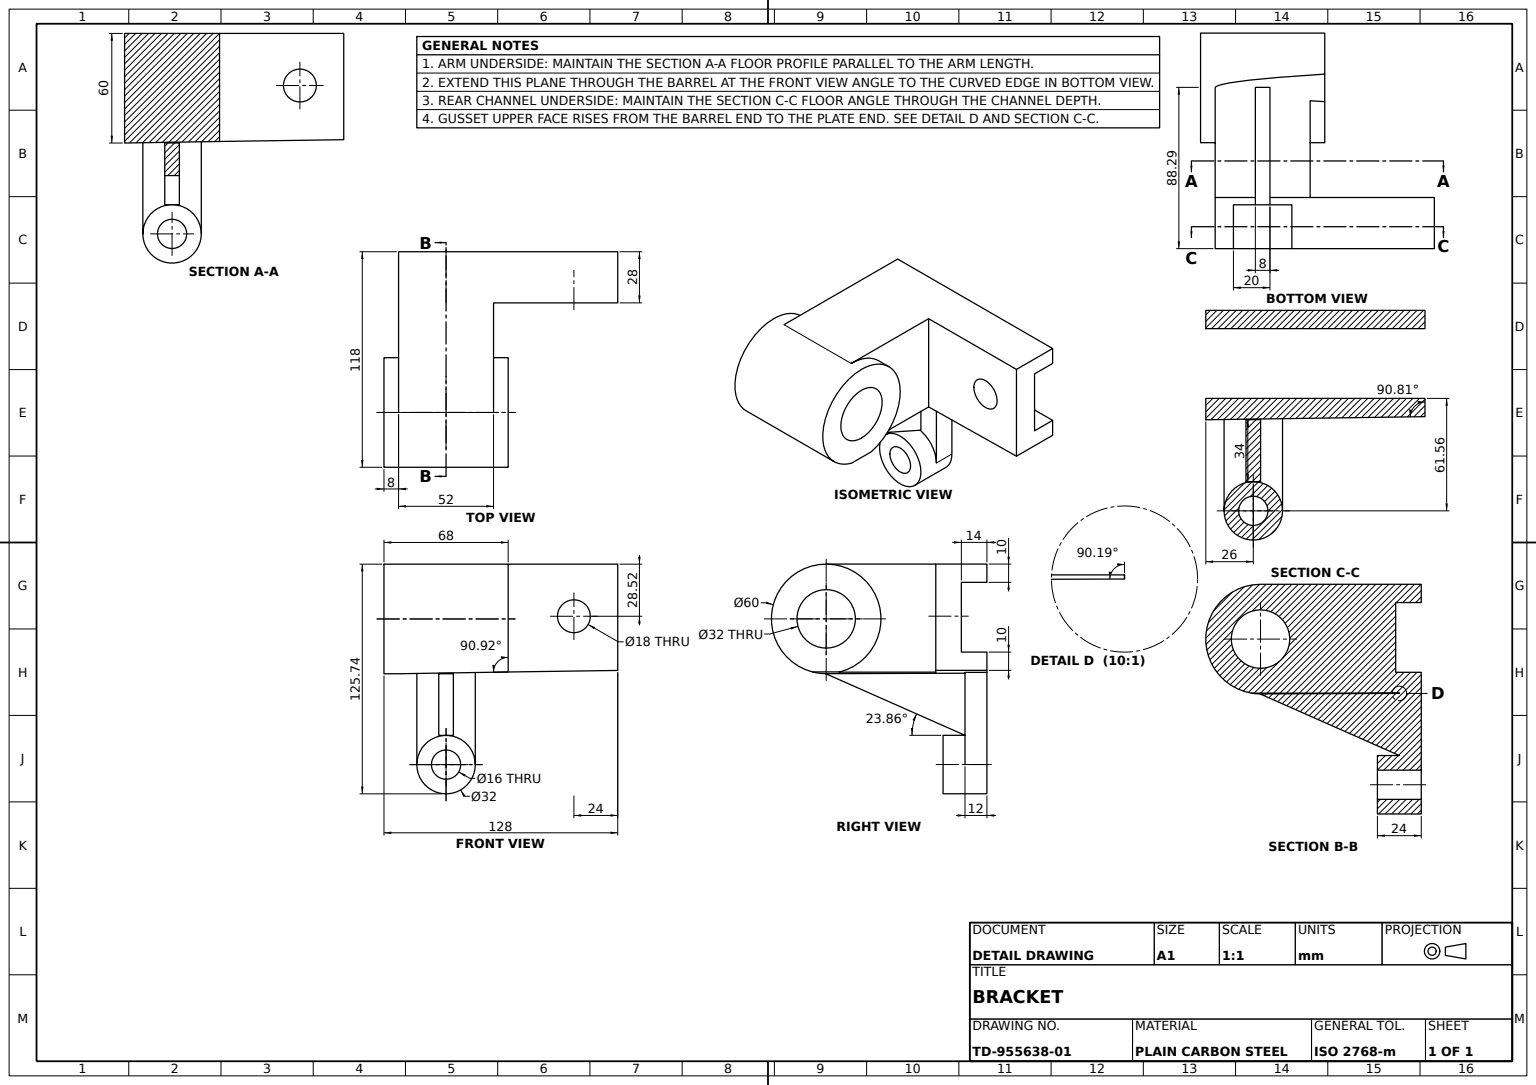
from build123d import *
from build123d.topology import SkipClean

# Parameters (mm, degrees)
BASE_BLOCK_DEPTH            = 28
UPRIGHT_WALL_SKETCH_W       = 60
UPRIGHT_WALL_SKETCH_H       = 60
UPRIGHT_WALL_DEPTH          = 68
BEARING_BOSS_SKETCH_R       = 30
BEARING_BOSS_60_DEPTH       = 68
BEARING_BORE_SKETCH_R       = 16
BEARING_BORE_32_DEPTH       = 68
BASE_PROFILE_CUT_DEPTH      = 128
THROUGH_HOLE_SKETCH_R       = 9
THROUGH_HOLE_18_DEPTH       = 128
END_START                   = -8
END_CHANNEL_RECESS_DEPTH    = 8
WALL_RECESS_DEPTH           = 8
TRIANGULAR_RELIEF_CUT_DEPTH = 100
SIDE_LUG_PLATE_DEPTH        = 12
LUG_BOSS_SKETCH_R           = 16
LUG_BOSS_32_DEPTH           = 12
LUG_GUSSET_DEPTH            = 20
GUSSET_TRIM_CUT_DEPTH       = 12
LUG_HOLE_SKETCH_R           = 8
LUG_HOLE_16_DEPTH           = 24


with BuildPart() as part:
    # Base Block Sketch → Base Block (new body)
    with BuildSketch(Plane.XY):
        Polygon((0, 0), (128, 1.815602837), (128, 60), (0, 60), align=None)
    extrude(amount=BASE_BLOCK_DEPTH)

    # Upright Wall Sketch → Upright Wall (add)
    with BuildSketch(Plane.ZY):
        with Locations((58, 30)):
            Rectangle(UPRIGHT_WALL_SKETCH_W, UPRIGHT_WALL_SKETCH_H)
    extrude(amount=-UPRIGHT_WALL_DEPTH)

    # Bearing Boss Sketch → Bearing Boss Ø60 (add)
    with BuildSketch(Plane(origin=(68, 0, 0), x_dir=(0, 0, -1), z_dir=(1, 0, 0))):
        with Locations((-88, 30)):
            Circle(BEARING_BOSS_SKETCH_R)
    extrude(amount=-BEARING_BOSS_60_DEPTH)

    # Bearing Bore Sketch → Bearing Bore Ø32 (cut)
    with BuildSketch(Plane(origin=(68, 0, 0), x_dir=(0, 0, -1), z_dir=(1, 0, 0))):
        with Locations(Location((-88, 30, 0), (0, 0, 90))):
            Circle(BEARING_BORE_SKETCH_R)
    extrude(amount=-BEARING_BORE_32_DEPTH, mode=Mode.SUBTRACT)

    # Base Profile Cut Sketch → Base Profile Cut (cut)
    with BuildSketch(Plane(origin=(128, 0, 0), x_dir=(0, 0, -1), z_dir=(1, 0, 0))):
        Polygon((0, 11.815602837), (0, 50), (-14, 50), (-14, 30.907801418), (-14, 11.815602837), align=None)
    extrude(amount=-BASE_PROFILE_CUT_DEPTH, mode=Mode.SUBTRACT)

    # Through Hole Sketch → Through Hole Ø18 (cut)
    with BuildSketch(Plane.XY.offset(28)):
        with Locations((104, 31.47819511)):
            Circle(THROUGH_HOLE_SKETCH_R)
    extrude(amount=-THROUGH_HOLE_18_DEPTH, mode=Mode.SUBTRACT)

    # End Channel Recess Sketch → End Channel Recess (cut)
    with SkipClean():  # the faces are left unmerged after this step: merging them gives an invalid solid
        with BuildSketch(Plane.ZY.offset(END_START)):
            with BuildLine():
                Line((0, 60), (88, 60))
                ThreePointArc((88, 60), (58, 30), (88, 0))
                Line((88, 0), (0, 0))
                Line((0, 0), (0, 11.815602837))
                Line((0, 11.815602837), (14, 11.815602837))
                Line((14, 11.815602837), (14, 50))
                Line((14, 50), (0, 50))
                Line((0, 50), (0, 60))
            make_face()
        extrude(amount=END_CHANNEL_RECESS_DEPTH, mode=Mode.SUBTRACT)

    # Wall Recess Sketch → Wall Recess (cut)
    with SkipClean():  # the faces are left unmerged after this step: merging them gives an invalid solid
        with BuildSketch(Plane(origin=(68, 0, 0), x_dir=(0, 0, -1), z_dir=(1, 0, 0))):
            with BuildLine():
                Line((-28, 60), (-28, 0))
                Line((-28, 0), (-88, 0))
                ThreePointArc((-88, 0), (-58, 30), (-88, 60))
                Line((-88, 60), (-28, 60))
            make_face()
        extrude(amount=-WALL_RECESS_DEPTH, mode=Mode.SUBTRACT)

    # Triangular Relief Sketch → Triangular Relief Cut (cut)
    with SkipClean():  # the faces are left unmerged after this step: merging them gives an invalid solid
        with BuildSketch(Plane(origin=(0, 0, 28), x_dir=(-1, 0, 0), z_dir=(0, 0, -1))):
            Polygon((-68, 0), (-68, 0.964539007), (-8, 0), align=None)
        extrude(amount=-TRIANGULAR_RELIEF_CUT_DEPTH, mode=Mode.SUBTRACT)

    # Side Lug Plate Sketch → Side Lug Plate (add)
    with SkipClean():  # the faces are left unmerged after this step: merging them gives an invalid solid
        with BuildSketch(Plane(origin=(0, 0, 0), x_dir=(-1, 0, 0), z_dir=(0, 0, -1))):
            with BuildLine():
                Line((-50, -49.744680851), (-50, 0.709219858))
                Line((-50, 0.709219858), (-18, 0.255319149))
                Line((-18, 0.255319149), (-18, -49.744680851))
                ThreePointArc((-18, -49.744680851), (-34, -65.744680851), (-50, -49.744680851))
            make_face()
        extrude(amount=-SIDE_LUG_PLATE_DEPTH)

    # Lug Boss Sketch → Lug Boss Ø32 (add)
    with SkipClean():  # the faces are left unmerged after this step: merging them gives an invalid solid
        with BuildSketch(Plane.XY.offset(12)):
            with Locations((34, -49.744680851)):
                Circle(LUG_BOSS_SKETCH_R)
        extrude(amount=LUG_BOSS_32_DEPTH)

    # Lug Gusset Sketch → Lug Gusset (add)
    with SkipClean():  # the faces are left unmerged after this step: merging them gives an invalid solid
        with BuildSketch(Plane(origin=(50, 0, 0), x_dir=(0, 0, -1), z_dir=(1, 0, 0))):
            Polygon((-12, 0.255319149), (-12, -33.744680851), (-88.292467077, 0), align=None)
        extrude(amount=-LUG_GUSSET_DEPTH)

    # Gusset Trim Sketch → Gusset Trim Cut (cut)
    with SkipClean():  # the faces are left unmerged after this step: merging them gives an invalid solid
        with BuildSketch(Plane(origin=(50, 0, 0), x_dir=(0, 0, -1), z_dir=(1, 0, 0))):
            Polygon((-88.292467077, 0), (-12, 0.255319149), (-12, -33.744680851), align=None)
        extrude(amount=-GUSSET_TRIM_CUT_DEPTH, mode=Mode.SUBTRACT)

    # Lug Hole Sketch → Lug Hole Ø16 (cut)
    with SkipClean():  # the faces are left unmerged after this step: merging them gives an invalid solid
        with BuildSketch(Plane.XY.offset(24)):
            with Locations((34, -49.744680851)):
                Circle(LUG_HOLE_SKETCH_R)
        extrude(amount=-LUG_HOLE_16_DEPTH, mode=Mode.SUBTRACT)


solid = part.part
